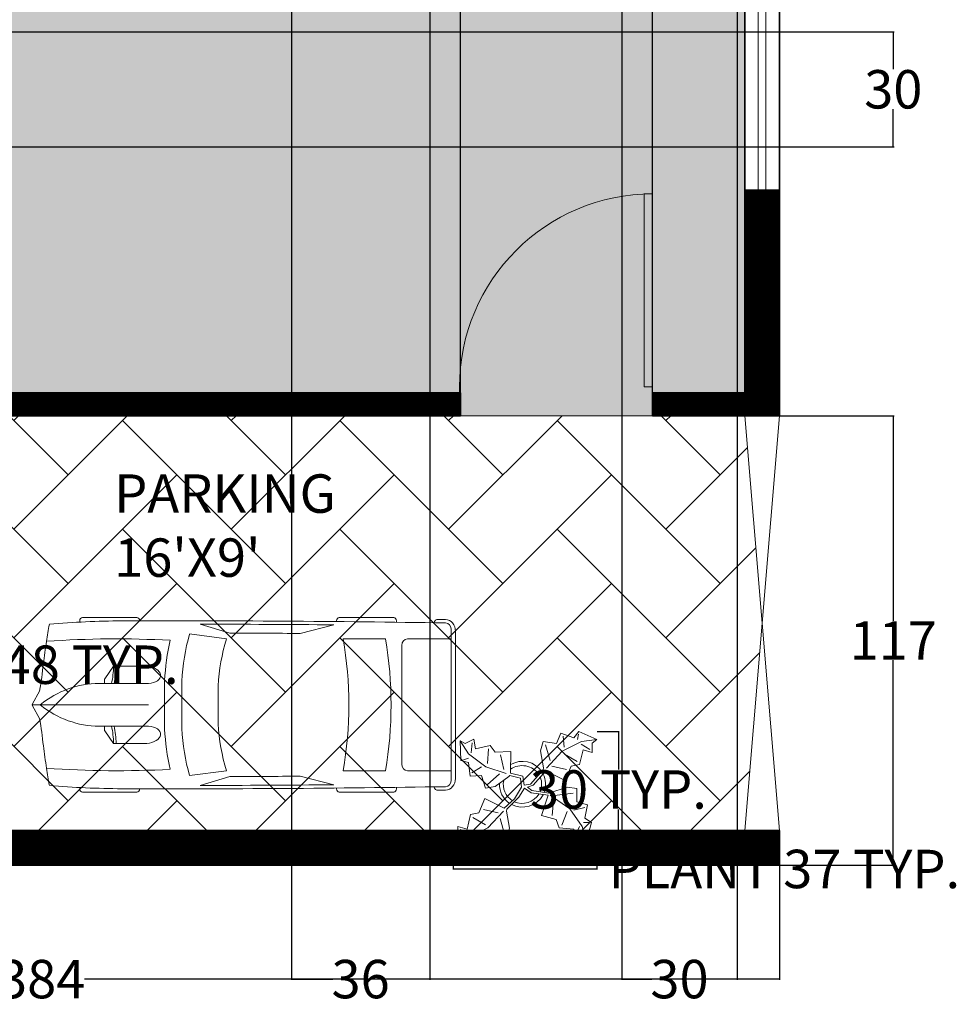
# Model space of a CAD drawing. Units: inches. Extents: x -89252 to 1164, y -183799 to 823.
# Tile 2 of 4: x 907 to 1150, y 159 to 416. Entities that reach past the tile are written whole.
import ezdxf

# ---------------------------------------------------------------- set-up
doc = ezdxf.new("R2010")
doc.units = ezdxf.units.IN
doc.header["$MEASUREMENT"] = 0
for name, color, linetype, lineweight in [('A-ANNO-DIMS', 2, 'Continuous', 18), ('A-AREA-IDEN', 7, 'Continuous', 25), ('A-GLAZ', 4, 'Continuous', 18), ('A-WALL', 7, 'Continuous', 35), ('CAR', 7, 'Continuous', 13), ('DOOR', 7, 'Continuous', 18), ('PLANT', 3, 'Continuous', 13)]:
    doc.layers.add(name, color=color, linetype=linetype, lineweight=lineweight)
for name, color, linetype, lineweight, true_color in [('A-FLOR-PATT', 252, 'Continuous', 13, 0x939598), ('A-WALL-PATT', 18, 'Continuous', 13, 0x000000), ('L-PVMT-PATT', 51, 'Continuous', 13, 0xf8f6b0)]:
    doc.layers.add(name, color=color, linetype=linetype, lineweight=lineweight, true_color=true_color)
doc.styles.get("Standard").update_dxf_attribs({"font": 'arial.ttf'})
doc.dimstyles.get("Standard").update_dxf_attribs({"dimtxt": 10, "dimasz": 0.18, "dimexe": 0.18, "dimexo": 0.0625, "dimgap": 0.09, "dimtad": 0, "dimtih": 1, "dimtoh": 1, "dimdec": 0, "dimzin": 0, "dimdsep": 46, "dimlunit": 3, "dimtxsty": 'Standard', "dimcen": 0.09, "dimadec": 0, "dimazin": 0, "dimtfac": 1, "dimtdec": 0, "dimtofl": 0, "dimtmove": 0, "dimatfit": 3, "dimfxl": 1, "dimtolj": 1, "dimtzin": 0, "dimarcsym": 0})

# ---------------------------------------------------------------- blocks, each defined once
blk = doc.blocks.new('*U10')
for p, q in [((0, 0), (0, -6)), ((-40, 0), (-40, -6))]:
    blk.add_line(p, q)
blk.add_lwpolyline([(0, 0), (0, 40), (-1.75, 40), (-1.75, 0)], close=True)
blk.add_arc((0, 0), 40, 90, 180)
blk = doc.blocks.new('*U14')
for p, q in [((21.1, 37.41), (21.1, 36.83)), ((46.55, 38.89), (22.35, 38.89)), ((47.8, 37.39), (47.8, 37.41)), ((87.99, 31.87), (74.76, 35.92)), ((134.31, 35.6), (119.29, 31.78)), ((135.45, 37.07), (135.45, 37.41)), ((136.7, 38.89), (160.9, 38.89)), ((162.15, 37.41), (162.15, 36.77)), ((70.03, 31.54), (86.41, 29.35)), ((186.47, -33.5), (186.47, 33.5)), ((188.4, -32.76), (188.4, 32.76)), ((138.42, 29.35), (157.25, 29.35)), ((164.52, 26.39), (164.52, -26.39)), ((186.47, 29.35), (167.01, 29.35)), ((32.27, 11.63), (36.13, 17.17)), ((36.13, 17.17), (50.94, 17.17)), ((29.77, 9.51), (51.68, 9.51)), ((32.12, 9.51), (32.12, 11.15)), ((58.92, -10.77), (58.92, 10.77)), ((66.55, -10.53), (66.55, 10.53)), ((186.47, -10.53), (186.47, 10.53)), ((3.27, 6.13), (0.1, 0.41)), ((82.74, 8.5), (82.74, -8.5)), ((0, 0), (51.68, 0)), ((0.1, -0.41), (3.27, -6.13)), ((29.77, -9.51), (51.68, -9.51)), ((32.12, -9.51), (32.12, -11.15)), ((32.27, -11.63), (36.13, -17.17)), ((36.13, -17.17), (50.94, -17.17)), ((86.41, -29.35), (70.03, -31.54)), ((157.25, -29.35), (138.42, -29.35)), ((167.01, -29.35), (186.47, -29.35)), ((87.99, -31.87), (74.76, -35.92)), ((134.31, -35.6), (119.29, -31.78)), ((21.1, -37.41), (21.1, -36.83)), ((46.55, -38.89), (22.35, -38.89)), ((47.8, -37.39), (47.8, -37.41)), ((135.45, -37.07), (135.45, -37.41)), ((136.7, -38.89), (160.9, -38.89)), ((162.15, -37.41), (162.15, -36.77))]:
    blk.add_line(p, q)
for centre, major_axis, ratio, start_param, end_param in [((266.03, -27.52), (0, 313.31), 0.842304, 1.367076, 1.39176), ((41.19, -490.86), (0, 528.23), 0.842304, 0.00281, 0.075598), ((22.35, 37.41), (0, -1.48), 0.842304, 3.141593, 4.712389), ((64.48, -10555.62), (0, 10593.03), 0.842304, -0.013397, 0.002797), ((46.55, 37.41), (0, 1.48), 0.842304, -1.570796, 0), ((64.48, -10555.62), (0, -10591.55), 0.842304, 3.133765, 3.140441), ((136.7, 37.41), (0, -1.48), 0.842304, 3.141593, 4.712389), ((160.9, 37.41), (0, 1.48), 0.842304, -1.570796, 0), ((180.63, 35.84), (0, 2.22), 0.842304, -0.013017, 1.249894), ((64.48, -10556.36), (0, 10595.31), 0.842304, -0.013397, -0.013017), ((183.98, 33.5), (0, -2.96), 0.842304, 1.570796, 3.128196), ((183.98, 32.76), (0, -5.25), 0.842304, 1.570796, 3.128196), ((135.29, 5.39), (0, 81.77), 0.842304, 1.245306, 1.50788), ((95.79, -3666.35), (0, -3698.24), 0.842304, 3.134049, 3.144098), ((259.18, -27.52), (0, -305.3), 0.842304, 4.528606, 4.561838), ((37.47, -593.96), (0, -623.33), 0.842304, 3.096046, 3.200911), ((134.4, 5.39), (0, -89.78), 0.842304, 4.449482, 4.652344), ((149.6, 2.8), (0, -79.58), 0.842304, 4.372215, 4.640744), ((17.08, 0), (0, 147.02), 0.842304, 4.511394, 4.913384), ((35.91, 0), (0, 147.02), 0.842304, 4.511394, 4.913384), ((167.01, 26.39), (0, 2.96), 0.842304, 0, 1.570796), ((-204.49, 52.4), (0, -250.96), 0.842304, 1.385369, 1.434372), ((13.04, 17.01), (0, 27.42), 0.842304, 4.435146, 4.718221), ((14.2, 17.01), (0, 27.42), 0.842304, 4.435146, 4.718221), ((50.79, 13.34), (6.34, -0.36), 0.603834, -1.395552, 1.581315), ((29.77, -46.66), (0, 56.17), 0.842304, 0, 0.590319), ((32.75, 11.15), (0, 0.74), 0.842304, 0.879714, 1.570796), ((0.62, 0), (0, -0.74), 0.842304, 4.131459, 5.293319), ((29.77, 46.66), (0, 56.17), 0.842304, 2.551274, 3.141593), ((-204.49, -52.4), (0, 250.96), 0.842304, -1.434372, -1.385369), ((149.6, -2.8), (0, -79.58), 0.842304, -1.499151, -1.230623), ((32.75, -11.15), (0, -0.74), 0.842304, 4.712389, 5.403472), ((13.04, -17.01), (0, -27.42), 0.842304, 1.564964, 1.848039), ((14.2, -17.01), (0, -27.42), 0.842304, 1.564964, 1.848039), ((134.4, -5.39), (0, -89.78), 0.842304, -1.510751, -1.307889), ((135.29, -5.39), (0, -81.77), 0.842304, -1.50788, -1.245306), ((259.18, 27.52), (0, 305.3), 0.842304, 1.721348, 1.754579), ((266.03, 27.52), (0, 313.31), 0.842304, 1.749832, 1.774517), ((37.47, 593.96), (0, -623.33), 0.842304, -0.059319, 0.045547), ((167.01, -26.39), (0, -2.96), 0.842304, 4.712389, 6.283185), ((95.79, 3666.35), (0, -3698.24), 0.842304, -0.002505, 0.007544), ((183.98, -33.5), (0, 2.96), 0.842304, 3.15499, 4.712389), ((183.98, -32.76), (0, -5.25), 0.842304, 0.013397, 1.570796), ((41.19, 490.86), (0, -528.23), 0.842304, -0.075598, -0.00281), ((22.35, -37.41), (0, 1.48), 0.842304, 1.570796, 3.141593), ((64.48, 10555.62), (0, 10593.03), 0.842304, 3.138796, 3.15499), ((46.55, -37.41), (0, -1.48), 0.842304, 0, 1.570796), ((64.48, 10555.62), (0, -10591.55), 0.842304, 0.001152, 0.007828), ((136.7, -37.41), (0, -1.48), 0.842304, -1.570796, 0), ((160.9, -37.41), (0, 1.48), 0.842304, 3.141593, 4.712389), ((180.63, -35.84), (0, -2.22), 0.842304, -1.249894, 0.013017), ((64.48, 10556.36), (0, 10595.31), 0.842304, 3.15461, 3.15499)]:
    blk.add_ellipse(centre, major_axis=major_axis, ratio=ratio, start_param=start_param, end_param=end_param)
at = {"extrusion": (0, 0, -1)}
blk.add_ellipse((50.79, -13.34), major_axis=(6.34, 0.36), ratio=0.603834, start_param=-1.395552, end_param=1.581315, dxfattribs=at)
blk = doc.blocks.new('Plant - Rubber or Philodendron')
for p, q in [((8.8871, 10.7908), (9.9809, 13.4933)), ((9.9809, 13.4933), (13.3837, 12.301)), ((13.3837, 12.301), (14.68, 13.9039)), ((14.5816, 13.2037), (14.3848, 11.8033)), ((14.68, 13.9039), (19.3848, 11.8146)), ((-16.2005, 11.4774), (-13.9899, 8.1064)), ((-16.2005, 11.4774), (-14.8639, 10.7964)), ((-16.0159, 6.3329), (-16.2005, 11.4774)), ((-14.8639, 10.7964), (-12.6195, 11.8975)), ((-13.3174, 8.325), (-13.0735, 11.0065)), ((-12.6195, 11.8975), (-12.1909, 9.4345)), ((-12.1909, 9.4345), (-8.3829, 10.3)), ((-8.3829, 10.3), (-7.0549, 8.501)), ((4.6914, 8.8812), (5.3859, 11.2828)), ((5.3859, 11.2828), (8.8871, 10.7908)), ((5.9878, 10.4842), (7.1971, 6.3869)), ((15.3859, 11.3055), (10.3916, 8.7942)), ((10.5828, 12.6946), (10.8893, 9.7953)), ((15.2875, 10.6053), (17.5907, 9.2105)), ((19.3848, 11.8146), (15.3859, 11.3055)), ((19.3848, 11.8146), (18.1868, 10.9119)), ((18.1868, 10.9119), (18.1925, 8.4119)), ((-13.9899, 8.1064), (-9.5434, 4.7185)), ((-8.8369, 9.409), (-9.0894, 5.6095)), ((-7.0549, 8.501), (-3.0284, 8.6941)), ((-4.8529, 4.012), (-5.7184, 7.82)), ((-3.0284, 8.6941), (-3.0709, 3.1041)), ((4.6914, 8.8812), (5.5014, 4.4831)), ((10.3916, 8.7942), (6.2847, 4.4028)), ((14.2977, 6.1031), (10.9934, 7.9956)), ((15.7909, 9.1065), (14.8995, 5.3044)), ((18.1925, 8.4119), (15.7909, 9.1065)), ((-14.0069, 5.8704), (-16.0159, 6.3329)), ((-15.3434, 6.5514), (-13.9984, 6.9884)), ((-13.5868, 2.2894), (-14.0069, 5.8704)), ((14.8995, 5.3044), (12.7005, 4.8994)), ((-13.1329, 3.1804), (-10.6614, 4.727)), ((-9.5434, 4.7185), (-4.1917, 2.9888)), ((-9.1318, 0.0195), (-5.9793, 2.9025)), ((-3.0709, 3.1041), (0.0797, 2.3163)), ((2.1141, 0.2298), (5.4346, 3.9146)), ((6.1032, 3.6844), (2.8262, -0.031)), ((5.4346, 3.9146), (5.5014, 4.4831)), ((11.1089, 1.1958), (6.1032, 3.6844)), ((7.7005, 4.8881), (11.5025, 3.9967)), ((12.7005, 4.8994), (11.1089, 1.1958)), ((-10.6784, 2.491), (-13.5868, 2.2894)), ((-9.5858, -0.8715), (-10.6784, 2.491)), ((-7.1228, -0.443), (-3.5248, 2.2131)), ((-3.5248, 2.2131), (-3.3011, 2.4355)), ((-3.3011, 2.4355), (-0.5306, 1.7947)), ((-0.5306, 1.7947), (-0.2255, -0.5527)), ((-0.5306, 1.7947), (-0.5306, 1.7947)), ((0.0797, 2.3163), (0.4866, -0.031)), ((0.4866, -0.031), (2.1141, 0.2298)), ((-7.1228, -0.443), (-9.5858, -0.8715)), ((-2.019, -3.6148), (-0.2255, -0.5527)), ((-0.9375, -3.1608), (0.5883, -0.8135)), ((0.5883, -0.8135), (2.2447, -2.0916)), ((2.8262, -0.031), (1.3003, -0.5527)), ((1.3003, -0.5527), (2.4193, -1.4655)), ((2.2447, -2.0916), (6.7108, -2.6626)), ((2.4193, -1.4655), (6.895, -2.1175)), ((11.6605, -0.5413), (6.895, -2.1175)), ((8.3544, -2.7453), (13.1973, -2.1704)), ((11.6605, -0.5413), (14.1354, -0.8948)), ((14.1354, -0.8948), (14.1354, -4.4304)), ((-11.3237, -7.2629), (-9.7321, -3.5593)), ((-9.7321, -3.5593), (-4.7264, -6.0479)), ((-2.019, -3.6148), (-4.7264, -6.0479)), ((-4.0579, -6.2781), (-0.9375, -3.1608)), ((4.943, -7.9659), (6.7108, -2.6626)), ((12.3677, -6.1981), (7.219, -2.6772)), ((8.125, -4.0768), (7.7715, -7.9659)), ((14.1354, -4.4304), (16.9638, -5.1375)), ((-14.4141, -11.4699), (-13.5228, -7.6679)), ((-13.5228, -7.6679), (-11.3237, -7.2629)), ((-6.3237, -7.2516), (-10.1257, -6.3602)), ((-9.0148, -11.1577), (-4.9047, -6.8122)), ((-4.1246, -6.8466), (-4.0579, -6.2781)), ((-3.3146, -11.2447), (-4.1246, -6.8466)), ((10.2463, -10.4408), (11.6605, -6.9053)), ((15.5496, -10.7943), (12.3677, -6.1981)), ((16.2567, -5.8446), (13.4283, -6.5517)), ((16.9638, -5.1375), (16.2567, -8.673)), ((-12.921, -8.4665), (-9.6166, -10.359)), ((-4.611, -12.8477), (-5.8203, -8.7504)), ((8.8321, -9.0266), (4.943, -7.9659)), ((9.5392, -11.1479), (8.8321, -9.0266)), ((17.3174, -9.7337), (15.9032, -9.7337)), ((16.2567, -8.673), (18.0245, -9.7337)), ((18.0245, -9.7337), (16.6103, -14.6834)), ((-16.8157, -10.7754), (-14.4141, -11.4699)), ((-16.8101, -13.2754), (-16.8157, -10.7754)), ((-13.9107, -12.9688), (-16.2139, -11.574)), ((-14.0091, -13.669), (-9.0148, -11.1577)), ((-9.206, -15.0581), (-9.5126, -12.1588)), ((-3.3146, -11.2447), (-4.0092, -13.6463)), ((13.4283, -11.5015), (9.5392, -11.1479)), ((13.0748, -13.9763), (13.4283, -11.5015)), ((14.8425, -10.7943), (13.7819, -13.2692)), ((16.6103, -14.6834), (15.5496, -10.7943)), ((-18.008, -14.1781), (-16.8101, -13.2754)), ((-18.008, -14.1781), (-14.0091, -13.669)), ((-13.3032, -16.2674), (-18.008, -14.1781)), ((-12.0069, -14.6645), (-13.3032, -16.2674)), ((-13.2048, -15.5672), (-13.008, -14.1668)), ((-8.6042, -15.8568), (-12.0069, -14.6645)), ((-7.5103, -13.1543), (-8.6042, -15.8568)), ((-4.0092, -13.6463), (-7.5103, -13.1543)), ((15.5496, -13.6228), (13.0748, -13.9763)), ((16.6103, -14.6834), (15.5496, -13.6228))]:
    blk.add_line(p, q)
for centre, radius, start, end in [((0, 0), 6.1275, 34.37569, 120.1028), ((-0.0601, -0.2075), 5.2461, 33.82192, 124.9414), ((-0.098, 0.1364), 6.1288, 341.2017, 26.09184), ((0.0308, 0.1664), 6, 178.6147, 235.1169), ((0.0308, 0.1664), 5, 168.1647, 238.6725), ((-0.2664, 0.1682), 5.2775, 338.4094, 20.03007), ((-0.1102, 0.4886), 5.2883, 247.3711, 327.472), ((-0.0234, 0.3825), 6.1492, 242.5812, 331.2714)]:
    blk.add_arc(centre, radius, start, end)
blk = doc.blocks.new('WIN-48IN-9IN-WALL')
for p, q in [((0, 48), (9, 48)), ((3.5, 0), (3.5, 48)), ((5.5, 0), (5.5, 48)), ((0, 0), (9, 0))]:
    blk.add_line(p, q)
blk = doc.blocks.new('*D22')
at = {"layer": 'A-ANNO-DIMS', "color": 0, "lineweight": -2, "transparency": 16777216}
for p, q in [((789.36, 240.45), (789.36, 247.77)), ((789.54, 247.59), (837.18, 247.59)), ((837.36, 240.45), (837.36, 247.77)), ((837.36, 247.59), (837.54, 247.59))]:
    blk.add_line(p, q, dxfattribs=at)
at = {"layer": 'A-ANNO-DIMS', "color": 0, "transparency": 16777216}
for points in [[(789.54, 247.62), (789.54, 247.56), (789.36, 247.59)], [(837.18, 247.62), (837.18, 247.56), (837.36, 247.59)]]:
    blk.add_solid(points, dxfattribs=at)
at = {"layer": 'Defpoints', "color": 0, "transparency": 16777216}
for p in [(837.36, 247.59), (789.36, 240.39), (837.36, 240.39)]:
    blk.add_point(p, dxfattribs=at)
at = {"layer": 'A-ANNO-DIMS', "color": 0, "transparency": 16777216, "insert": (894.77, 247.59), "char_height": 10, "attachment_point": 5}
blk.add_mtext('\\A1;WINDOW 48 TYP.', dxfattribs=at)
blk = doc.blocks.new('*D26')
at = {"layer": 'A-ANNO-DIMS', "color": 0, "lineweight": -2, "transparency": 16777216}
for p, q in [((1019.46, 199.95), (1019.46, 194.23)), ((1056.85, 199.95), (1056.85, 194.23)), ((1019.64, 194.41), (1056.67, 194.41)), ((1056.85, 194.41), (1057.03, 194.41))]:
    blk.add_line(p, q, dxfattribs=at)
at = {"layer": 'A-ANNO-DIMS', "color": 0, "transparency": 16777216}
for points in [[(1019.64, 194.44), (1019.64, 194.38), (1019.46, 194.41)], [(1056.67, 194.44), (1056.67, 194.38), (1056.85, 194.41)]]:
    blk.add_solid(points, dxfattribs=at)
at = {"layer": 'Defpoints', "color": 0, "transparency": 16777216}
for p in [(1019.46, 200.02), (1056.85, 200.02), (1056.85, 194.41)]:
    blk.add_point(p, dxfattribs=at)
at = {"layer": 'A-ANNO-DIMS', "color": 0, "transparency": 16777216, "insert": (1105.66, 194.41), "char_height": 10, "attachment_point": 5}
blk.add_mtext('\\A1;PLANT 37 TYP.', dxfattribs=at)
blk = doc.blocks.new('*D27')
at = {"layer": 'A-ANNO-DIMS', "color": 0, "lineweight": -2, "transparency": 16777216}
for p, q in [((1056.91, 230.19), (1062.64, 230.19)), ((1062.46, 230.01), (1062.46, 220.3)), ((1062.46, 200.2), (1062.46, 209.9)), ((1056.91, 200.02), (1062.64, 200.02))]:
    blk.add_line(p, q, dxfattribs=at)
at = {"layer": 'A-ANNO-DIMS', "color": 0, "transparency": 16777216}
for points in [[(1062.43, 230.01), (1062.49, 230.01), (1062.46, 230.19)], [(1062.43, 200.2), (1062.49, 200.2), (1062.46, 200.02)]]:
    blk.add_solid(points, dxfattribs=at)
at = {"layer": 'Defpoints', "color": 0, "transparency": 16777216}
for p in [(1056.85, 230.19), (1062.46, 230.19), (1056.85, 200.02)]:
    blk.add_point(p, dxfattribs=at)
at = {"layer": 'A-ANNO-DIMS', "color": 0, "transparency": 16777216, "insert": (1062.46, 215.1), "char_height": 10, "attachment_point": 5}
blk.add_mtext('\\A1;30 TYP.', dxfattribs=at)
blk = doc.blocks.new('*D30')
at = {"layer": 'A-ANNO-DIMS', "color": 0, "lineweight": -2, "transparency": 16777216}
for p, q in [((720.36, 195.33), (720.36, 165.56)), ((1104.36, 195.33), (1104.36, 165.56)), ((720.54, 165.74), (901.25, 165.74)), ((1104.18, 165.74), (923.48, 165.74))]:
    blk.add_line(p, q, dxfattribs=at)
at = {"layer": 'A-ANNO-DIMS', "color": 0, "transparency": 16777216}
for points in [[(720.54, 165.77), (720.54, 165.71), (720.36, 165.74)], [(1104.18, 165.77), (1104.18, 165.71), (1104.36, 165.74)]]:
    blk.add_solid(points, dxfattribs=at)
at = {"layer": 'Defpoints', "color": 0, "transparency": 16777216}
for p in [(720.36, 195.39), (1104.36, 195.39), (1104.36, 165.74)]:
    blk.add_point(p, dxfattribs=at)
at = {"layer": 'A-ANNO-DIMS', "color": 0, "transparency": 16777216, "insert": (912.36, 165.74), "char_height": 10, "attachment_point": 5}
blk.add_mtext('\\A1;384', dxfattribs=at)
blk = doc.blocks.new('*D32')
at = {"layer": 'A-ANNO-DIMS', "color": 0, "lineweight": -2, "transparency": 16777216}
for p, q in [((1104.43, 312.39), (1134.19, 312.39)), ((1134.01, 312.21), (1134.01, 259)), ((1134.01, 195.57), (1134.01, 248.78)), ((1104.43, 195.39), (1134.19, 195.39))]:
    blk.add_line(p, q, dxfattribs=at)
at = {"layer": 'A-ANNO-DIMS', "color": 0, "transparency": 16777216}
for points in [[(1133.98, 312.21), (1134.04, 312.21), (1134.01, 312.39)], [(1133.98, 195.57), (1134.04, 195.57), (1134.01, 195.39)]]:
    blk.add_solid(points, dxfattribs=at)
at = {"layer": 'Defpoints', "color": 0, "transparency": 16777216}
for p in [(1104.36, 312.39), (1134.01, 312.39), (1104.36, 195.39)]:
    blk.add_point(p, dxfattribs=at)
at = {"layer": 'A-ANNO-DIMS', "color": 0, "transparency": 16777216, "insert": (1134.01, 253.89), "char_height": 10, "attachment_point": 5}
blk.add_mtext('\\A1;117', dxfattribs=at)
blk = doc.blocks.new('*D34')
at = {"layer": 'A-ANNO-DIMS', "color": 0, "lineweight": -2, "transparency": 16777216}
for p, q in [((1021.36, 318.45), (1021.36, 816.22)), ((1021.54, 816.04), (1039.13, 816.04)), ((1071.18, 816.04), (1053.6, 816.04)), ((1071.36, 318.45), (1071.36, 816.22))]:
    blk.add_line(p, q, dxfattribs=at)
at = {"layer": 'A-ANNO-DIMS', "color": 0, "transparency": 16777216}
for points in [[(1021.54, 816.07), (1021.54, 816.01), (1021.36, 816.04)], [(1071.18, 816.07), (1071.18, 816.01), (1071.36, 816.04)]]:
    blk.add_solid(points, dxfattribs=at)
at = {"layer": 'Defpoints', "color": 0, "transparency": 16777216}
for p in [(1071.36, 816.04), (1021.36, 318.39), (1071.36, 318.39)]:
    blk.add_point(p, dxfattribs=at)
at = {"layer": 'A-ANNO-DIMS', "color": 0, "transparency": 16777216, "insert": (1046.36, 816.04), "char_height": 10, "attachment_point": 5}
blk.add_mtext('\\A1;50', dxfattribs=at)
blk = doc.blocks.new('*D39')
at = {"layer": 'A-ANNO-DIMS', "color": 0, "lineweight": -2, "transparency": 16777216}
for p, q in [((977.36, 564.33), (977.36, 165.56)), ((1013.36, 564.33), (1013.36, 165.56)), ((977.54, 165.74), (988.12, 165.74)), ((1013.18, 165.74), (1002.61, 165.74))]:
    blk.add_line(p, q, dxfattribs=at)
at = {"layer": 'A-ANNO-DIMS', "color": 0, "transparency": 16777216}
for points in [[(977.54, 165.77), (977.54, 165.71), (977.36, 165.74)], [(1013.18, 165.77), (1013.18, 165.71), (1013.36, 165.74)]]:
    blk.add_solid(points, dxfattribs=at)
at = {"layer": 'Defpoints', "color": 0, "transparency": 16777216}
for p in [(977.36, 564.39), (1013.36, 564.39), (1013.36, 165.74)]:
    blk.add_point(p, dxfattribs=at)
at = {"layer": 'A-ANNO-DIMS', "color": 0, "transparency": 16777216, "insert": (995.36, 165.74), "char_height": 10, "attachment_point": 5}
blk.add_mtext('\\A1;36', dxfattribs=at)
blk = doc.blocks.new('*D40')
at = {"layer": 'A-ANNO-DIMS', "color": 0, "lineweight": -2, "transparency": 16777216}
for p, q in [((1063.36, 672.33), (1063.36, 165.56)), ((1093.36, 672.33), (1093.36, 165.56)), ((1063.54, 165.74), (1071.13, 165.74)), ((1093.18, 165.74), (1085.6, 165.74))]:
    blk.add_line(p, q, dxfattribs=at)
at = {"layer": 'A-ANNO-DIMS', "color": 0, "transparency": 16777216}
for points in [[(1063.54, 165.77), (1063.54, 165.71), (1063.36, 165.74)], [(1093.18, 165.77), (1093.18, 165.71), (1093.36, 165.74)]]:
    blk.add_solid(points, dxfattribs=at)
at = {"layer": 'Defpoints', "color": 0, "transparency": 16777216}
for p in [(1063.36, 672.39), (1093.36, 672.39), (1093.36, 165.74)]:
    blk.add_point(p, dxfattribs=at)
at = {"layer": 'A-ANNO-DIMS', "color": 0, "transparency": 16777216, "insert": (1078.36, 165.74), "char_height": 10, "attachment_point": 5}
blk.add_mtext('\\A1;30', dxfattribs=at)
blk = doc.blocks.new('*D46')
at = {"layer": 'A-ANNO-DIMS', "color": 0, "lineweight": -2, "transparency": 16777216}
for p, q in [((1071.36, 318.45), (1071.36, 816.22)), ((1071.54, 816.04), (1076.05, 816.04)), ((1095.18, 816.04), (1090.68, 816.04)), ((1095.36, 318.45), (1095.36, 816.22))]:
    blk.add_line(p, q, dxfattribs=at)
at = {"layer": 'A-ANNO-DIMS', "color": 0, "transparency": 16777216}
for points in [[(1071.54, 816.07), (1071.54, 816.01), (1071.36, 816.04)], [(1095.18, 816.07), (1095.18, 816.01), (1095.36, 816.04)]]:
    blk.add_solid(points, dxfattribs=at)
at = {"layer": 'Defpoints', "color": 0, "transparency": 16777216}
for p in [(1095.36, 816.04), (1071.36, 318.39), (1095.36, 318.39)]:
    blk.add_point(p, dxfattribs=at)
at = {"layer": 'A-ANNO-DIMS', "color": 0, "transparency": 16777216, "insert": (1083.36, 816.04), "char_height": 10, "attachment_point": 5}
blk.add_mtext('\\A1;24', dxfattribs=at)
blk = doc.blocks.new('*D55')
at = {"layer": 'A-ANNO-DIMS', "color": 0, "lineweight": -2, "transparency": 16777216}
for p, q in [((897.43, 412.39), (1134.19, 412.39)), ((1134.01, 412.21), (1134.01, 402.59)), ((1134.01, 382.57), (1134.01, 392.19)), ((897.43, 382.39), (1134.19, 382.39))]:
    blk.add_line(p, q, dxfattribs=at)
at = {"layer": 'A-ANNO-DIMS', "color": 0, "transparency": 16777216}
for points in [[(1133.98, 412.21), (1134.04, 412.21), (1134.01, 412.39)], [(1133.98, 382.57), (1134.04, 382.57), (1134.01, 382.39)]]:
    blk.add_solid(points, dxfattribs=at)
at = {"layer": 'Defpoints', "color": 0, "transparency": 16777216}
for p in [(897.36, 412.39), (1134.01, 412.39), (897.36, 382.39)]:
    blk.add_point(p, dxfattribs=at)
at = {"layer": 'A-ANNO-DIMS', "color": 0, "transparency": 16777216, "insert": (1134.01, 397.39), "char_height": 10, "attachment_point": 5}
blk.add_mtext('\\A1;30', dxfattribs=at)

msp = doc.modelspace()

# ---------------------------------------------------------------- hatches: boundary and pattern name
at = {"layer": 'A-FLOR-PATT'}
h = msp.add_hatch(color=256, dxfattribs=at)
h.dxf.hatch_style = 1
h.paths.add_polyline_path([(1095.364, 558.3893), (1013.364, 558.3893), (1013.364, 564.3893), (1095.364, 564.3893), (1095.364, 672.3893), (1093.364, 672.3893), (1063.364, 672.3893), (1005.364, 672.3893), (1005.364, 726.3893), (975.364, 726.3893), (975.364, 690.3893), (975.364, 564.3893), (977.364, 564.3893), (977.364, 558.3893), (975.364, 558.3893), (969.364, 558.3893), (967.364, 558.3893), (967.364, 564.3893), (969.364, 564.3893), (969.364, 684.3893), (967.364, 684.3893), (937.364, 684.3893), (891.364, 684.3893), (891.364, 588.3893), (929.3053, 588.3893), (929.3053, 564.3893), (937.364, 564.3893), (937.364, 558.3893), (857.364, 558.3893), (857.364, 564.3893), (861.364, 564.3893), (861.364, 684.3893), (729.364, 684.3893), (729.364, 564.3893), (781.364, 564.3893), (781.364, 558.3893), (729.364, 558.3893), (729.364, 510.3893), (813.364, 510.3893), (813.364, 558.3893), (811.364, 558.3893), (811.364, 564.3893), (813.364, 564.3893), (819.364, 564.3893), (821.364, 564.3893), (821.364, 558.3893), (819.364, 558.3893), (819.364, 510.3893), (859.364, 510.3893), (859.364, 420.3893), (903.364, 420.3893), (903.364, 414.3893), (903.364, 412.3893), (897.364, 412.3893), (897.364, 414.3893), (813.364, 414.3893), (813.364, 366.3893), (897.364, 366.3893), (897.364, 382.3893), (903.364, 382.3893), (903.364, 360.3893), (903.364, 358.3893), (897.364, 358.3893), (897.364, 360.3893), (807.364, 360.3893), (805.364, 360.3893), (805.364, 366.3893), (807.364, 366.3893), (807.364, 414.3893), (729.364, 414.3893), (729.364, 366.3893), (775.364, 366.3893), (775.364, 360.3893), (729.364, 360.3893), (729.364, 240.3893), (897.364, 240.3893), (897.364, 318.3893), (1021.364, 318.3893), (1021.364, 312.3893), (1071.364, 312.3893), (1071.364, 318.3893), (1095.364, 318.3893)])
h.paths.add_polyline_path([(1095.364, 726.3893), (1011.364, 726.3893), (1011.364, 678.3893), (1063.364, 678.3893), (1063.364, 672.3893), (1093.364, 672.3893), (1093.364, 678.3893), (1095.364, 678.3893)])
h.paths.add_polyline_path([(969.364, 726.3893), (729.364, 726.3893), (729.364, 690.3893), (937.364, 690.3893), (937.364, 684.3893), (967.364, 684.3893), (967.364, 690.3893), (969.364, 690.3893)])
at = {"layer": 'A-WALL-PATT'}
h = msp.add_hatch(dxfattribs=at)
h.set_pattern_fill('ANSI31', color=256)
h.paths.add_polyline_path([(867.364, 684.3893), (878.364, 684.3893), (878.364, 690.3893), (817.6735, 690.3893), (817.6735, 684.3893), (861.364, 684.3893), (861.364, 564.3893), (857.364, 564.3893), (857.364, 558.3893), (937.364, 558.3893), (937.364, 564.3893), (867.364, 564.3893)], flags=17)
h.paths.add_polyline_path([(1041.364, 735.3893), (720.364, 735.3893), (720.364, 546.3893), (729.364, 546.3893), (729.364, 558.3893), (781.364, 558.3893), (781.364, 564.3893), (729.364, 564.3893), (729.364, 684.3893), (769.6735, 684.3893), (769.6735, 690.3893), (729.364, 690.3893), (729.364, 726.3893), (969.364, 726.3893), (969.364, 690.3893), (967.364, 690.3893), (967.364, 684.3893), (969.364, 684.3893), (969.364, 564.3893), (967.364, 564.3893), (967.364, 558.3893), (969.364, 558.3893), (975.364, 558.3893), (977.364, 558.3893), (977.364, 564.3893), (975.364, 564.3893), (975.364, 690.3893), (975.364, 726.3893), (1005.364, 726.3893), (1005.364, 672.3893), (1063.364, 672.3893), (1063.364, 678.3893), (1011.364, 678.3893), (1011.364, 726.3893), (1041.364, 726.3893)])
h.paths.add_polyline_path([(1104.364, 735.3893), (1065.364, 735.3893), (1065.364, 726.3893), (1095.364, 726.3893), (1095.364, 678.3893), (1093.364, 678.3893), (1093.364, 672.3893), (1095.364, 672.3893), (1095.364, 642.3893), (1104.364, 642.3893)])
h.paths.add_polyline_path([(1104.364, 594.3893), (1095.364, 594.3893), (1095.364, 564.3893), (1013.364, 564.3893), (1013.364, 558.3893), (1095.364, 558.3893), (1095.364, 515.2697), (1104.364, 515.2697)])
h.paths.add_polyline_path([(1104.364, 467.2697), (1095.364, 467.2697), (1095.364, 419.2348), (1104.364, 419.2348)])
h.paths.add_polyline_path([(1104.364, 371.2348), (1095.364, 371.2348), (1095.364, 312.3893), (1104.364, 312.3893)], flags=17)
h.paths.add_polyline_path([(1095.364, 318.3893), (1071.364, 318.3893), (1071.364, 312.3893), (1095.364, 312.3893)], flags=17)
h.paths.add_polyline_path([(1021.364, 318.3893), (897.364, 318.3893), (897.364, 240.3893), (837.364, 240.3893), (837.364, 234.3893), (903.364, 234.3893), (903.364, 312.3893), (1021.364, 312.3893)], flags=17)
h.paths.add_polyline_path([(903.364, 382.3893), (897.364, 382.3893), (897.364, 366.3893), (813.364, 366.3893), (813.364, 414.3893), (897.364, 414.3893), (897.364, 412.3893), (903.364, 412.3893), (903.364, 414.3893), (903.364, 420.3893), (729.364, 420.3893), (729.364, 504.3893), (859.364, 504.3893), (859.364, 510.3893), (819.364, 510.3893), (819.364, 558.3893), (821.364, 558.3893), (821.364, 564.3893), (819.364, 564.3893), (813.364, 564.3893), (811.364, 564.3893), (811.364, 558.3893), (813.364, 558.3893), (813.364, 510.3893), (729.364, 510.3893), (729.364, 522.3893), (720.364, 522.3893), (720.364, 400.5349), (729.364, 400.5349), (729.364, 414.3893), (807.364, 414.3893), (807.364, 366.3893), (805.364, 366.3893), (805.364, 360.3893), (807.364, 360.3893), (897.364, 360.3893), (897.364, 358.3893), (903.364, 358.3893), (903.364, 360.3893)])
h.paths.add_polyline_path([(775.364, 366.3893), (729.364, 366.3893), (729.364, 376.5349), (720.364, 376.5349), (720.364, 195.3893), (1104.364, 195.3893), (1104.364, 204.3893), (729.364, 204.3893), (729.364, 234.3893), (789.364, 234.3893), (789.364, 240.3893), (729.364, 240.3893), (729.364, 360.3893), (775.364, 360.3893)])
h.paths.add_polyline_path([(937.364, 690.3893), (926.364, 690.3893), (926.364, 684.3893), (937.364, 684.3893)], flags=17)
at = {"layer": 'L-PVMT-PATT'}
h = msp.add_hatch(dxfattribs=at)
h.set_pattern_fill('AR-HBONE', color=256, scale=5)
h.paths.add_polyline_path([(1099.864, 258.3893), (1095.364, 312.3893), (1071.364, 312.3893), (1021.364, 312.3893), (903.364, 312.3893), (903.364, 234.3893), (729.364, 234.3893), (729.364, 204.3893), (1095.364, 204.3893)])

# ---------------------------------------------------------------- linework, layer by layer
at = {"layer": 'A-WALL'}
for p, q in [((1104.364, 312.3893), (1104.364, 735.3893)), ((1095.364, 312.3893), (1095.364, 558.3893)), ((897.364, 318.3893), (1021.364, 318.3893)), ((1021.364, 312.3893), (1021.364, 318.3893)), ((1071.364, 312.3893), (1071.364, 318.3893)), ((1071.364, 318.3893), (1095.364, 318.3893)), ((903.364, 312.3893), (1021.364, 312.3893)), ((1071.364, 312.3893), (1104.364, 312.3893)), ((729.364, 204.3893), (1104.364, 204.3893)), ((1104.364, 195.3893), (1104.364, 204.3893)), ((720.364, 195.3893), (1104.364, 195.3893))]:
    msp.add_line(p, q, dxfattribs=at)
at = {"layer": 'DOOR'}
for p, q in [((1021.364, 312.3893), (1071.364, 312.3893)), ((1095.364, 312.3893), (1104.364, 204.3893)), ((1095.364, 204.3893), (1104.364, 312.3893))]:
    msp.add_line(p, q, dxfattribs=at)

# ---------------------------------------------------------------- block references
at = {"layer": 'A-GLAZ', "rotation": 180}
msp.add_blockref('WIN-48IN-9IN-WALL', (1104.3641, 419.2351), dxfattribs=at)
at = {"layer": 'CAR', "xscale": 0.5845354604094469, "yscale": 0.5845354604094469, "zscale": 0.5845354604094469}
msp.add_blockref('*U14', (909.9141, 237.1476), dxfattribs=at)
at = {"layer": 'DOOR', "xscale": 1.256154847611548, "yscale": 1.256154847611548, "zscale": 1.256154847611548}
msp.add_blockref('*U10', (1071.364, 319.9263), dxfattribs=at)
at = {"layer": 'PLANT'}
msp.add_blockref('Plant - Rubber or Philodendron', (1037.4658, 216.2846), dxfattribs=at)

# ---------------------------------------------------------------- texts
at = {"layer": 'A-AREA-IDEN', "insert": (931.2198, 297.1387), "char_height": 10, "attachment_point": 1}
msp.add_mtext_dynamic_manual_height_columns("PARKING\\P16'X9'", width=99.889598, gutter_width=1, heights=[0], dxfattribs=at)

# ---------------------------------------------------------------- dimensions: what is measured, and where the dimension line sits
at = {"layer": 'A-ANNO-DIMS'}
for base, p1, p2, picture, middle in [((1071.364, 816.0393), (1021.364, 318.3893), (1071.364, 318.3893), '*D34', (1046.364, 816.0393)), ((1095.364, 816.0393), (1071.364, 318.3893), (1095.364, 318.3893), '*D46', (1083.364, 816.0393)), ((1093.364, 165.7393), (1063.364, 672.3893), (1093.364, 672.3893), '*D40', (1078.364, 165.7393)), ((1013.364, 165.7393), (977.364, 564.3893), (1013.364, 564.3893), '*D39', (995.364, 165.7393)), ((1104.364, 165.7393), (720.364, 195.3893), (1104.364, 195.3893), '*D30', (912.364, 165.7393))]:
    dim = msp.add_linear_dim(base=base, p1=p1, p2=p2, dimstyle='Standard', override={"dimdec": 0, "dimlfac": 1, "dimrnd": 0, "dimzin": 0, "dimdsep": 46, "dimlunit": 2}, dxfattribs=at)
    dim.commit()
    dim.dimension.update_dxf_attribs({"geometry": picture, "text_midpoint": middle})
for base, p1, p2, picture, middle in [((1134.014, 412.3893), (897.364, 382.3893), (897.364, 412.3893), '*D55', (1134.014, 397.3893)), ((1134.014, 312.3893), (1104.364, 195.3893), (1104.364, 312.3893), '*D32', (1134.014, 253.8893))]:
    dim = msp.add_linear_dim(base=base, p1=p1, p2=p2, angle=90, dimstyle='Standard', override={"dimdec": 0, "dimlfac": 1, "dimrnd": 0, "dimzin": 0, "dimdsep": 46, "dimlunit": 2}, dxfattribs=at)
    dim.commit()
    dim.dimension.update_dxf_attribs({"geometry": picture, "text_midpoint": middle})
for base, p1, p2, text, picture, middle in [((837.364, 247.5893), (789.364, 240.3893), (837.364, 240.3893), 'WINDOW <> TYP.', '*D22', (894.7657, 247.5893)), ((1056.8506, 194.4083), (1019.4578, 200.0172), (1056.8506, 200.0172), 'PLANT <> TYP.', '*D26', (1105.6643, 194.4083))]:
    dim = msp.add_linear_dim(base=base, p1=p1, p2=p2, text=text, dimstyle='Standard', override={"dimdec": 0, "dimlfac": 1, "dimrnd": 0, "dimzin": 0, "dimdsep": 46, "dimlunit": 2}, dxfattribs=at)
    dim.commit()
    dim.dimension.update_dxf_attribs({"geometry": picture, "text_midpoint": middle})
dim = msp.add_linear_dim(base=(1062.4595, 230.1885), p1=(1056.8506, 200.0172), p2=(1056.8506, 230.1885), angle=90, text='<> TYP.', dimstyle='Standard', override={"dimdec": 0, "dimlfac": 1, "dimrnd": 0, "dimzin": 0, "dimdsep": 46, "dimlunit": 2}, dxfattribs=at)
dim.commit()
dim.dimension.update_dxf_attribs({"geometry": '*D27', "text_midpoint": (1062.4595, 215.1028)})

doc.saveas('drawing.dxf')
